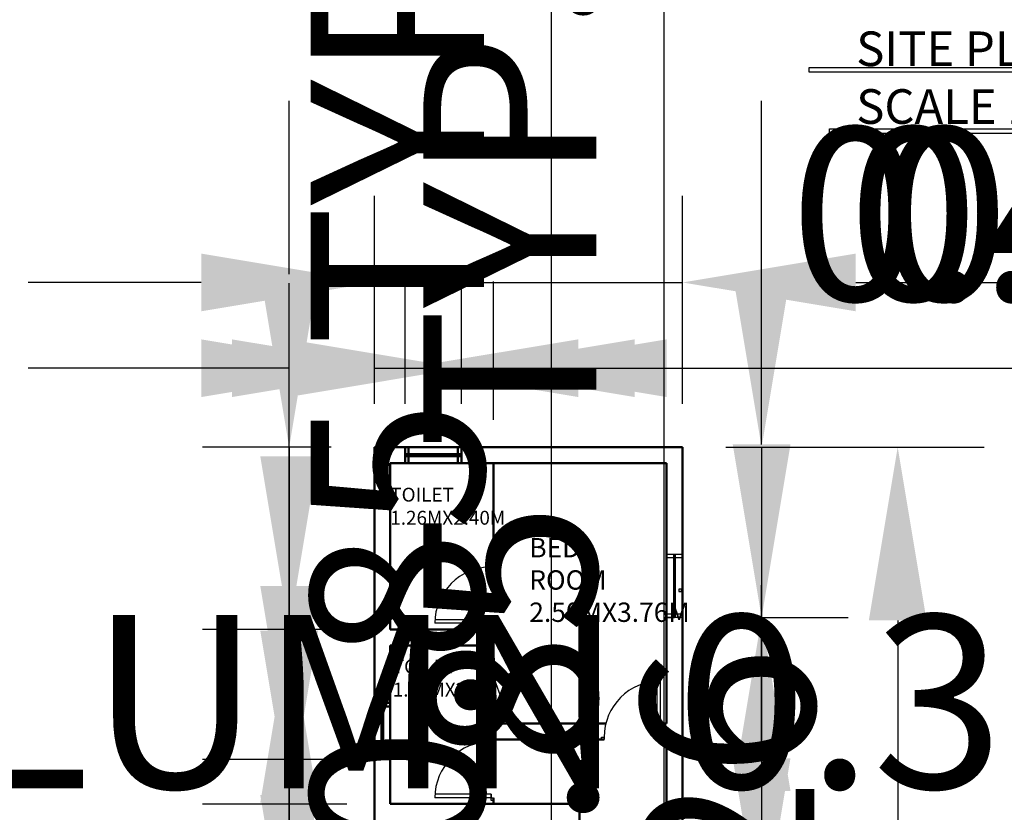
# Model space of a CAD drawing. Units: metres. Extents: x 782 to 1487, y 1262 to 7446.
# Tile 7 of 25: x 807.01 to 821.23, y 1302.06 to 1313.5. Entities that reach past the tile are written whole.
import ezdxf

# ---------------------------------------------------------------- set-up
doc = ezdxf.new("R2010")
doc.units = ezdxf.units.M
for name, color, linetype, lineweight in [('A-ANNO-DIMS', 2, 'Continuous', 18), ('A-ANNO-TEXT', 3, 'Continuous', 18), ('A-AREA-IDEN', 3, 'Continuous', 18), ('A-DOOR', 4, 'Continuous', 25), ('A-GLAZ', 4, 'Continuous', 25), ('A-WALL', 7, 'Continuous', 50), ('C-PROP', 6, 'Continuous', 25)]:
    doc.layers.add(name, color=color, linetype=linetype, lineweight=lineweight)
doc.styles.get("Standard").update_dxf_attribs({"font": 'arial.ttf'})
doc.dimstyles.new('ISO-25', dxfattribs={"dimtxt": 2.5, "dimasz": 2.5, "dimexe": 1.25, "dimexo": 0.625, "dimtad": 1, "dimtxsty": 'Standard', "dimcen": 2.5, "dimadec": 0, "dimazin": 0, "dimtfac": 1, "dimtmove": 0, "dimatfit": 3, "dimfxl": 1, "dimarcsym": 0})

# ---------------------------------------------------------------- blocks, each defined once
blk = doc.blocks.new('*D4')
at = {"layer": 'A-ANNO-DIMS', "color": 0, "lineweight": -2, "transparency": 16777216}
for p, q in [((817.205, 1307.327), (820.936, 1307.327)), ((819.686, 1304.827), (819.686, 1295.567)), ((817.205, 1293.067), (820.936, 1293.067))]:
    blk.add_line(p, q, dxfattribs=at)
at = {"layer": 'A-ANNO-DIMS', "color": 0, "transparency": 16777216}
for points in [[(819.269, 1304.827), (820.103, 1304.827), (819.686, 1307.327)], [(819.269, 1295.567), (820.103, 1295.567), (819.686, 1293.067)]]:
    blk.add_solid(points, dxfattribs=at)
at = {"layer": 'Defpoints', "color": 0, "transparency": 16777216}
for p in [(816.58, 1307.327), (816.58, 1293.067), (819.686, 1293.067)]:
    blk.add_point(p, dxfattribs=at)
at = {"layer": 'A-ANNO-DIMS', "color": 0, "transparency": 16777216, "insert": (817.558, 1300.197), "char_height": 2.5, "attachment_point": 5, "rotation": 90}
blk.add_mtext('14,26', dxfattribs=at)
blk = doc.blocks.new('*D5')
at = {"layer": 'A-ANNO-DIMS', "color": 0, "lineweight": -2, "transparency": 16777216}
for p, q in [((812.13, 1307.952), (812.13, 1310.955)), ((816.58, 1307.952), (816.58, 1310.955)), ((809.63, 1309.705), (807.13, 1309.705)), ((812.13, 1309.705), (816.58, 1309.705)), ((819.08, 1309.705), (829.443, 1309.705))]:
    blk.add_line(p, q, dxfattribs=at)
at = {"layer": 'A-ANNO-DIMS', "color": 0, "transparency": 16777216}
for points in [[(809.63, 1310.122), (809.63, 1309.289), (812.13, 1309.705)], [(819.08, 1310.122), (819.08, 1309.289), (816.58, 1309.705)]]:
    blk.add_solid(points, dxfattribs=at)
at = {"layer": 'Defpoints', "color": 0, "transparency": 16777216}
for p in [(816.58, 1309.705), (812.13, 1307.327), (816.58, 1307.327)]:
    blk.add_point(p, dxfattribs=at)
at = {"layer": 'A-ANNO-DIMS', "color": 0, "transparency": 16777216, "insert": (825.512, 1311.828), "char_height": 2.5, "attachment_point": 5}
blk.add_mtext('4,45', dxfattribs=at)
blk = doc.blocks.new('DOOR-810')
for p, q in [((0.813, 0.089), (0, 0.089)), ((0.813, 0.038), (0.813, 0.089))]:
    blk.add_line(p, q)
for points in [[(0.813, 0.851), (0.846, 0.851), (0.846, 0.89), (0.813, 0.89)], [(0.813, 0.038), (0.847, 0.038), (0.847, 0), (0.813, 0)]]:
    blk.add_lwpolyline(points, close=True)
blk.add_lwpolyline([(0.813, 0.089), (0.813, 0.038), (0, 0.038)])
blk.add_arc((0.813, 0.038), 0.813, 90, 180)
blk = doc.blocks.new('DOOR-810-C')
for p, q in [((0.801, 0.034), (0.801, 0.847)), ((0.851, 0.034), (0.801, 0.034))]:
    blk.add_line(p, q)
blk.add_lwpolyline([(0.801, 0.034), (0.851, 0.034), (0.851, 0.847)])
for points in [[(0.039, 0.034), (0.039, 0.002), (0, 0.002), (0, 0.034)], [(0.851, 0.034), (0.851, 0), (0.889, 0), (0.889, 0.034)]]:
    blk.add_lwpolyline(points, close=True)
blk.add_arc((0.851, 0.034), 0.813, 90, 180)
blk = doc.blocks.new('WIN-900-B')
for p, q in [((0, 0), (0, 0.914)), ((0, 0.914), (0.23, 0.914)), ((0.23, 0.863), (0, 0.863)), ((0.103, 0), (0.103, 0.914)), ((0.115, 0), (0.115, 0.914)), ((0.128, 0), (0.128, 0.914)), ((0.23, 0.914), (0.23, 0)), ((0.23, 0.914), (0.23, 0.863)), ((0.23, 0.051), (0, 0.051)), ((0.23, 0), (0.23, 0.051)), ((0.23, 0), (0, 0)), ((0, 0), (0.115, 0))]:
    blk.add_line(p, q)
blk.add_lwpolyline([(0.215, 0.379), (0.215, 0.412), (0.176, 0.412), (0.176, 0.379)], close=True)
blk = doc.blocks.new('*D23')
at = {"layer": 'A-ANNO-DIMS', "color": 0, "lineweight": -2, "transparency": 16777216}
for p, q in [((816.313, 1296.414), (816.313, 1315.246)), ((816.313, 1293.067), (816.313, 1293.914)), ((816.804, 1293.914), (817.563, 1293.914)), ((816.804, 1293.067), (817.563, 1293.067)), ((816.313, 1290.567), (816.313, 1288.067))]:
    blk.add_line(p, q, dxfattribs=at)
at = {"layer": 'A-ANNO-DIMS', "color": 0, "transparency": 16777216}
for points in [[(815.896, 1296.414), (816.729, 1296.414), (816.313, 1293.914)], [(815.896, 1290.567), (816.729, 1290.567), (816.313, 1293.067)]]:
    blk.add_solid(points, dxfattribs=at)
at = {"layer": 'Defpoints', "color": 0, "transparency": 16777216}
for p in [(816.179, 1293.914), (816.313, 1293.914), (816.179, 1293.067)]:
    blk.add_point(p, dxfattribs=at)
at = {"layer": 'A-ANNO-DIMS', "color": 0, "transparency": 16777216, "insert": (814.411, 1307.08), "char_height": 2.5, "attachment_point": 5, "rotation": 90}
blk.add_mtext('0.85 TYP.', dxfattribs=at)
blk = doc.blocks.new('*D24')
at = {"layer": 'A-ANNO-DIMS', "color": 0, "lineweight": -2, "transparency": 16777216}
for p, q in [((811.209, 1294.423), (808.709, 1294.423)), ((813.709, 1294.423), (814.559, 1294.423)), ((817.059, 1294.423), (852.649, 1294.423)), ((813.709, 1293.926), (813.709, 1293.173)), ((814.559, 1293.926), (814.559, 1293.173))]:
    blk.add_line(p, q, dxfattribs=at)
at = {"layer": 'A-ANNO-DIMS', "color": 0, "transparency": 16777216}
for points in [[(811.209, 1294.84), (811.209, 1294.006), (813.709, 1294.423)], [(817.059, 1294.84), (817.059, 1294.006), (814.559, 1294.423)]]:
    blk.add_solid(points, dxfattribs=at)
at = {"layer": 'Defpoints', "color": 0, "transparency": 16777216}
for p in [(813.709, 1294.551), (814.559, 1294.551), (814.559, 1294.423)]:
    blk.add_point(p, dxfattribs=at)
at = {"layer": 'A-ANNO-DIMS', "color": 0, "transparency": 16777216, "insert": (836.104, 1296.342), "char_height": 2.5, "attachment_point": 5}
blk.add_mtext('DOOR D2 0.85 TYP.', dxfattribs=at)
blk = doc.blocks.new('*D25')
at = {"layer": 'A-ANNO-DIMS', "color": 0, "lineweight": -2, "transparency": 16777216}
for p, q in [((814.687, 1297.897), (814.687, 1316.729)), ((814.687, 1294.551), (814.687, 1295.397)), ((815.184, 1295.397), (815.937, 1295.397)), ((815.184, 1294.551), (815.937, 1294.551)), ((814.687, 1292.051), (814.687, 1289.551))]:
    blk.add_line(p, q, dxfattribs=at)
at = {"layer": 'A-ANNO-DIMS', "color": 0, "transparency": 16777216}
for points in [[(814.27, 1297.897), (815.103, 1297.897), (814.687, 1295.397)], [(814.27, 1292.051), (815.103, 1292.051), (814.687, 1294.551)]]:
    blk.add_solid(points, dxfattribs=at)
at = {"layer": 'Defpoints', "color": 0, "transparency": 16777216}
for p in [(814.559, 1295.397), (814.687, 1295.397), (814.559, 1294.551)]:
    blk.add_point(p, dxfattribs=at)
at = {"layer": 'A-ANNO-DIMS', "color": 0, "transparency": 16777216, "insert": (812.785, 1308.563), "char_height": 2.5, "attachment_point": 5, "rotation": 90}
blk.add_mtext('0.85 TYP.', dxfattribs=at)
blk = doc.blocks.new('*D26')
at = {"layer": 'A-ANNO-DIMS', "color": 0, "lineweight": -2, "transparency": 16777216}
for p, q in [((828.33, 1303.223), (828.33, 1342.718)), ((828.33, 1299.809), (828.33, 1300.723)), ((828.818, 1300.723), (829.58, 1300.723)), ((828.818, 1299.809), (829.58, 1299.809)), ((828.33, 1297.309), (828.33, 1294.809))]:
    blk.add_line(p, q, dxfattribs=at)
at = {"layer": 'A-ANNO-DIMS', "color": 0, "transparency": 16777216}
for points in [[(827.913, 1303.223), (828.747, 1303.223), (828.33, 1300.723)], [(827.913, 1297.309), (828.747, 1297.309), (828.33, 1299.809)]]:
    blk.add_solid(points, dxfattribs=at)
at = {"layer": 'Defpoints', "color": 0, "transparency": 16777216}
for p in [(828.193, 1300.723), (828.33, 1300.723), (828.193, 1299.809)]:
    blk.add_point(p, dxfattribs=at)
at = {"layer": 'A-ANNO-DIMS', "color": 0, "transparency": 16777216, "insert": (826.412, 1324.22), "char_height": 2.5, "attachment_point": 5, "rotation": 90}
blk.add_mtext('WINDOW W 0.91 TYP.', dxfattribs=at)
blk = doc.blocks.new('*D30')
at = {"layer": 'A-ANNO-DIMS', "color": 0, "lineweight": -2, "transparency": 16777216}
for p, q in [((792.059, 1301.411), (789.559, 1301.411)), ((794.559, 1301.411), (794.946, 1301.411)), ((797.446, 1301.411), (832.354, 1301.411)), ((794.559, 1300.844), (794.559, 1300.161)), ((794.946, 1300.844), (794.946, 1300.161))]:
    blk.add_line(p, q, dxfattribs=at)
at = {"layer": 'A-ANNO-DIMS', "color": 0, "transparency": 16777216}
for points in [[(792.059, 1301.827), (792.059, 1300.994), (794.559, 1301.411)], [(797.446, 1301.827), (797.446, 1300.994), (794.946, 1301.411)]]:
    blk.add_solid(points, dxfattribs=at)
at = {"layer": 'Defpoints', "color": 0, "transparency": 16777216}
for p in [(794.559, 1301.469), (794.946, 1301.469), (794.946, 1301.411)]:
    blk.add_point(p, dxfattribs=at)
at = {"layer": 'A-ANNO-DIMS', "color": 0, "transparency": 16777216, "insert": (816.15, 1303.33), "char_height": 2.5, "attachment_point": 5}
blk.add_mtext('COLUMN 0.39 TYP.', dxfattribs=at)
blk = doc.blocks.new('*D43')
at = {"layer": 'A-ANNO-DIMS', "color": 0, "lineweight": -2, "transparency": 16777216}
for p, q in [((792.559, 1313.575), (792.559, 1315.72)), ((794.559, 1311.575), (794.559, 1315.72)), ((790.059, 1314.47), (787.559, 1314.47)), ((792.559, 1314.47), (794.559, 1314.47)), ((797.059, 1314.47), (807.337, 1314.47))]:
    blk.add_line(p, q, dxfattribs=at)
at = {"layer": 'A-ANNO-DIMS', "color": 0, "transparency": 16777216}
for points in [[(790.059, 1314.887), (790.059, 1314.054), (792.559, 1314.47)], [(797.059, 1314.887), (797.059, 1314.054), (794.559, 1314.47)]]:
    blk.add_solid(points, dxfattribs=at)
at = {"layer": 'Defpoints', "color": 0, "transparency": 16777216}
for p in [(794.559, 1314.47), (792.559, 1312.95), (794.559, 1310.95)]:
    blk.add_point(p, dxfattribs=at)
at = {"layer": 'A-ANNO-DIMS', "color": 0, "transparency": 16777216, "insert": (803.448, 1316.372), "char_height": 2.5, "attachment_point": 5}
blk.add_mtext('2.00', dxfattribs=at)
blk = doc.blocks.new('*D44')
at = {"layer": 'A-ANNO-DIMS', "color": 0, "lineweight": -2, "transparency": 16777216}
for p, q in [((800.039, 1311.575), (800.039, 1315.72)), ((801.429, 1313.575), (801.429, 1315.72)), ((797.539, 1314.47), (795.039, 1314.47)), ((800.039, 1314.47), (801.429, 1314.47)), ((803.929, 1314.47), (813.943, 1314.47))]:
    blk.add_line(p, q, dxfattribs=at)
at = {"layer": 'A-ANNO-DIMS', "color": 0, "transparency": 16777216}
for points in [[(797.539, 1314.887), (797.539, 1314.054), (800.039, 1314.47)], [(803.929, 1314.887), (803.929, 1314.054), (801.429, 1314.47)]]:
    blk.add_solid(points, dxfattribs=at)
at = {"layer": 'Defpoints', "color": 0, "transparency": 16777216}
for p in [(801.429, 1314.47), (801.429, 1312.95), (800.039, 1310.95)]:
    blk.add_point(p, dxfattribs=at)
at = {"layer": 'A-ANNO-DIMS', "color": 0, "transparency": 16777216, "insert": (810.186, 1316.373), "char_height": 2.5, "attachment_point": 5}
blk.add_mtext('1.39', dxfattribs=at)
blk = doc.blocks.new('*D53')
at = {"layer": 'A-ANNO-DIMS', "color": 0, "lineweight": -2, "transparency": 16777216}
for p, q in [((810.9, 1309.827), (810.9, 1312.327)), ((811.505, 1307.327), (809.65, 1307.327)), ((810.9, 1307.327), (810.9, 1304.697)), ((811.735, 1304.697), (809.65, 1304.697)), ((810.9, 1302.197), (810.9, 1291.911))]:
    blk.add_line(p, q, dxfattribs=at)
at = {"layer": 'A-ANNO-DIMS', "color": 0, "transparency": 16777216}
for points in [[(810.483, 1309.827), (811.317, 1309.827), (810.9, 1307.327)], [(810.483, 1302.197), (811.317, 1302.197), (810.9, 1304.697)]]:
    blk.add_solid(points, dxfattribs=at)
at = {"layer": 'Defpoints', "color": 0, "transparency": 16777216}
for p in [(812.13, 1307.327), (810.9, 1304.697), (812.36, 1304.697)]:
    blk.add_point(p, dxfattribs=at)
at = {"layer": 'A-ANNO-DIMS', "color": 0, "transparency": 16777216, "insert": (808.998, 1295.804), "char_height": 2.5, "attachment_point": 5, "rotation": 90}
blk.add_mtext('2.63', dxfattribs=at)
blk = doc.blocks.new('*D54')
at = {"layer": 'A-ANNO-DIMS', "color": 0, "lineweight": -2, "transparency": 16777216}
for p, q in [((810.9, 1307.197), (810.9, 1309.697)), ((811.735, 1304.697), (809.65, 1304.697)), ((810.9, 1304.697), (810.9, 1302.822)), ((811.503, 1302.822), (809.65, 1302.822)), ((810.9, 1300.322), (810.9, 1290.308))]:
    blk.add_line(p, q, dxfattribs=at)
at = {"layer": 'A-ANNO-DIMS', "color": 0, "transparency": 16777216}
for points in [[(810.483, 1307.197), (811.317, 1307.197), (810.9, 1304.697)], [(810.483, 1300.322), (811.317, 1300.322), (810.9, 1302.822)]]:
    blk.add_solid(points, dxfattribs=at)
at = {"layer": 'Defpoints', "color": 0, "transparency": 16777216}
for p in [(812.36, 1304.697), (810.9, 1302.822), (812.128, 1302.822)]:
    blk.add_point(p, dxfattribs=at)
at = {"layer": 'A-ANNO-DIMS', "color": 0, "transparency": 16777216, "insert": (808.999, 1294.065), "char_height": 2.5, "attachment_point": 5, "rotation": 90}
blk.add_mtext('1.88', dxfattribs=at)
blk = doc.blocks.new('*D55')
at = {"layer": 'A-ANNO-DIMS', "color": 0, "lineweight": -2, "transparency": 16777216}
for p, q in [((810.9, 1305.322), (810.9, 1307.822)), ((811.503, 1302.822), (809.65, 1302.822)), ((810.9, 1302.822), (810.9, 1302.177)), ((811.735, 1302.177), (809.65, 1302.177)), ((810.9, 1299.677), (810.9, 1289.444))]:
    blk.add_line(p, q, dxfattribs=at)
at = {"layer": 'A-ANNO-DIMS', "color": 0, "transparency": 16777216}
for points in [[(810.483, 1305.322), (811.317, 1305.322), (810.9, 1302.822)], [(810.483, 1299.677), (811.317, 1299.677), (810.9, 1302.177)]]:
    blk.add_solid(points, dxfattribs=at)
at = {"layer": 'Defpoints', "color": 0, "transparency": 16777216}
for p in [(812.128, 1302.822), (810.9, 1302.177), (812.36, 1302.177)]:
    blk.add_point(p, dxfattribs=at)
at = {"layer": 'A-ANNO-DIMS', "color": 0, "transparency": 16777216, "insert": (808.999, 1293.311), "char_height": 2.5, "attachment_point": 5, "rotation": 90}
blk.add_mtext('0.64', dxfattribs=at)
blk = doc.blocks.new('*D56')
at = {"layer": 'A-ANNO-DIMS', "color": 0, "lineweight": -2, "transparency": 16777216}
for p, q in [((810.9, 1304.677), (810.9, 1307.177)), ((811.735, 1302.177), (809.65, 1302.177)), ((810.9, 1302.177), (810.9, 1299.809)), ((811.505, 1299.809), (809.65, 1299.809)), ((810.9, 1297.309), (810.9, 1287.022))]:
    blk.add_line(p, q, dxfattribs=at)
at = {"layer": 'A-ANNO-DIMS', "color": 0, "transparency": 16777216}
for points in [[(810.483, 1304.677), (811.317, 1304.677), (810.9, 1302.177)], [(810.483, 1297.309), (811.317, 1297.309), (810.9, 1299.809)]]:
    blk.add_solid(points, dxfattribs=at)
at = {"layer": 'Defpoints', "color": 0, "transparency": 16777216}
for p in [(812.36, 1302.177), (810.9, 1299.809), (812.13, 1299.809)]:
    blk.add_point(p, dxfattribs=at)
at = {"layer": 'A-ANNO-DIMS', "color": 0, "transparency": 16777216, "insert": (808.998, 1290.916), "char_height": 2.5, "attachment_point": 5, "rotation": 90}
blk.add_mtext('2.37', dxfattribs=at)
blk = doc.blocks.new('*D57')
at = {"layer": 'A-ANNO-DIMS', "color": 0, "lineweight": -2, "transparency": 16777216}
for p, q in [((810.9, 1302.309), (810.9, 1304.809)), ((811.505, 1299.809), (809.65, 1299.809)), ((810.9, 1299.809), (810.9, 1298.647)), ((811.735, 1298.647), (809.65, 1298.647)), ((810.9, 1296.147), (810.9, 1286.141))]:
    blk.add_line(p, q, dxfattribs=at)
at = {"layer": 'A-ANNO-DIMS', "color": 0, "transparency": 16777216}
for points in [[(810.483, 1302.309), (811.317, 1302.309), (810.9, 1299.809)], [(810.483, 1296.147), (811.317, 1296.147), (810.9, 1298.647)]]:
    blk.add_solid(points, dxfattribs=at)
at = {"layer": 'Defpoints', "color": 0, "transparency": 16777216}
for p in [(812.13, 1299.809), (810.9, 1298.647), (812.36, 1298.647)]:
    blk.add_point(p, dxfattribs=at)
at = {"layer": 'A-ANNO-DIMS', "color": 0, "transparency": 16777216, "insert": (808.999, 1289.894), "char_height": 2.5, "attachment_point": 5, "rotation": 90}
blk.add_mtext('1.16', dxfattribs=at)
blk = doc.blocks.new('*D58')
at = {"layer": 'A-ANNO-DIMS', "color": 0, "lineweight": -2, "transparency": 16777216}
for p, q in [((810.9, 1301.147), (810.9, 1303.647)), ((811.735, 1298.647), (809.65, 1298.647)), ((810.9, 1298.647), (810.9, 1296.5)), ((811.507, 1296.5), (809.65, 1296.5)), ((810.9, 1294), (810.9, 1281.772))]:
    blk.add_line(p, q, dxfattribs=at)
at = {"layer": 'A-ANNO-DIMS', "color": 0, "transparency": 16777216}
for points in [[(810.483, 1301.147), (811.317, 1301.147), (810.9, 1298.647)], [(810.483, 1294), (811.317, 1294), (810.9, 1296.5)]]:
    blk.add_solid(points, dxfattribs=at)
at = {"layer": 'Defpoints', "color": 0, "transparency": 16777216}
for p in [(812.36, 1298.647), (810.9, 1296.5), (812.132, 1296.5)]:
    blk.add_point(p, dxfattribs=at)
at = {"layer": 'A-ANNO-DIMS', "color": 0, "transparency": 16777216, "insert": (809.02, 1286.636), "char_height": 2.5, "attachment_point": 5, "rotation": 90}
blk.add_mtext('2.147', dxfattribs=at)
blk = doc.blocks.new('*D63')
at = {"layer": 'A-ANNO-DIMS', "color": 0, "lineweight": -2, "transparency": 16777216}
for p, q in [((817.721, 1309.827), (817.721, 1312.327)), ((817.205, 1307.327), (818.971, 1307.327)), ((817.721, 1307.327), (817.721, 1304.867)), ((817.205, 1304.867), (818.971, 1304.867)), ((817.721, 1302.367), (817.721, 1292.082))]:
    blk.add_line(p, q, dxfattribs=at)
at = {"layer": 'A-ANNO-DIMS', "color": 0, "transparency": 16777216}
for points in [[(817.304, 1309.827), (818.138, 1309.827), (817.721, 1307.327)], [(817.304, 1302.367), (818.138, 1302.367), (817.721, 1304.867)]]:
    blk.add_solid(points, dxfattribs=at)
at = {"layer": 'Defpoints', "color": 0, "transparency": 16777216}
for p in [(816.58, 1307.327), (816.58, 1304.867), (817.721, 1304.867)]:
    blk.add_point(p, dxfattribs=at)
at = {"layer": 'A-ANNO-DIMS', "color": 0, "transparency": 16777216, "insert": (815.82, 1295.974), "char_height": 2.5, "attachment_point": 5, "rotation": 90}
blk.add_mtext('2.46', dxfattribs=at)
blk = doc.blocks.new('*D64')
at = {"layer": 'A-ANNO-DIMS', "color": 0, "lineweight": -2, "transparency": 16777216}
for p, q in [((817.721, 1307.367), (817.721, 1309.867)), ((817.205, 1304.867), (818.971, 1304.867)), ((817.721, 1304.867), (817.721, 1300.338)), ((817.206, 1300.338), (818.971, 1300.338)), ((817.721, 1297.838), (817.721, 1285.546))]:
    blk.add_line(p, q, dxfattribs=at)
at = {"layer": 'A-ANNO-DIMS', "color": 0, "transparency": 16777216}
for points in [[(817.304, 1307.367), (818.138, 1307.367), (817.721, 1304.867)], [(817.304, 1297.838), (818.138, 1297.838), (817.721, 1300.338)]]:
    blk.add_solid(points, dxfattribs=at)
at = {"layer": 'Defpoints', "color": 0, "transparency": 16777216}
for p in [(816.58, 1304.867), (816.581, 1300.338), (817.721, 1300.338)]:
    blk.add_point(p, dxfattribs=at)
at = {"layer": 'A-ANNO-DIMS', "color": 0, "transparency": 16777216, "insert": (815.82, 1290.442), "char_height": 2.5, "attachment_point": 5, "rotation": 90}
blk.add_mtext('4.529', dxfattribs=at)
blk = doc.blocks.new('*D65')
at = {"layer": 'A-ANNO-DIMS', "color": 0, "lineweight": -2, "transparency": 16777216}
for p, q in [((817.721, 1302.838), (817.721, 1305.338)), ((817.206, 1300.338), (818.971, 1300.338)), ((817.721, 1300.338), (817.721, 1296.196)), ((817.205, 1296.196), (818.971, 1296.196)), ((817.721, 1293.696), (817.721, 1281.435))]:
    blk.add_line(p, q, dxfattribs=at)
at = {"layer": 'A-ANNO-DIMS', "color": 0, "transparency": 16777216}
for points in [[(817.304, 1302.838), (818.138, 1302.838), (817.721, 1300.338)], [(817.304, 1293.696), (818.138, 1293.696), (817.721, 1296.196)]]:
    blk.add_solid(points, dxfattribs=at)
at = {"layer": 'Defpoints', "color": 0, "transparency": 16777216}
for p in [(816.581, 1300.338), (816.58, 1296.196), (817.721, 1296.196)]:
    blk.add_point(p, dxfattribs=at)
at = {"layer": 'A-ANNO-DIMS', "color": 0, "transparency": 16777216, "insert": (815.841, 1286.315), "char_height": 2.5, "attachment_point": 5, "rotation": 90}
blk.add_mtext('4.142', dxfattribs=at)
blk = doc.blocks.new('*D70')
at = {"layer": 'A-ANNO-DIMS', "color": 0, "lineweight": -2, "transparency": 16777216}
for p, q in [((812.13, 1307.952), (812.13, 1309.718)), ((812.573, 1307.953), (812.573, 1309.718)), ((809.63, 1308.468), (807.13, 1308.468)), ((812.13, 1308.468), (812.573, 1308.468)), ((815.073, 1308.468), (825.307, 1308.468))]:
    blk.add_line(p, q, dxfattribs=at)
at = {"layer": 'A-ANNO-DIMS', "color": 0, "transparency": 16777216}
for points in [[(809.63, 1308.884), (809.63, 1308.051), (812.13, 1308.468)], [(815.073, 1308.884), (815.073, 1308.051), (812.573, 1308.468)]]:
    blk.add_solid(points, dxfattribs=at)
at = {"layer": 'Defpoints', "color": 0, "transparency": 16777216}
for p in [(812.573, 1308.468), (812.13, 1307.327), (812.573, 1307.328)]:
    blk.add_point(p, dxfattribs=at)
at = {"layer": 'A-ANNO-DIMS', "color": 0, "transparency": 16777216, "insert": (821.44, 1310.369), "char_height": 2.5, "attachment_point": 5}
blk.add_mtext('0.44', dxfattribs=at)
blk = doc.blocks.new('*D71')
at = {"layer": 'A-ANNO-DIMS', "color": 0, "lineweight": -2, "transparency": 16777216}
for p, q in [((812.573, 1307.953), (812.573, 1309.718)), ((813.387, 1307.953), (813.387, 1309.718)), ((810.073, 1308.468), (807.573, 1308.468)), ((812.573, 1308.468), (813.387, 1308.468)), ((815.887, 1308.468), (828.063, 1308.468))]:
    blk.add_line(p, q, dxfattribs=at)
at = {"layer": 'A-ANNO-DIMS', "color": 0, "transparency": 16777216}
for points in [[(810.073, 1308.884), (810.073, 1308.051), (812.573, 1308.468)], [(815.887, 1308.884), (815.887, 1308.051), (813.387, 1308.468)]]:
    blk.add_solid(points, dxfattribs=at)
at = {"layer": 'Defpoints', "color": 0, "transparency": 16777216}
for p in [(813.387, 1308.468), (812.573, 1307.328), (813.387, 1307.328)]:
    blk.add_point(p, dxfattribs=at)
at = {"layer": 'A-ANNO-DIMS', "color": 0, "transparency": 16777216, "insert": (823.225, 1310.369), "char_height": 2.5, "attachment_point": 5}
blk.add_mtext('0.814', dxfattribs=at)
blk = doc.blocks.new('*D72')
at = {"layer": 'A-ANNO-DIMS', "color": 0, "lineweight": -2, "transparency": 16777216}
for p, q in [((813.387, 1307.953), (813.387, 1309.718)), ((813.85, 1307.722), (813.85, 1309.718)), ((810.887, 1308.468), (808.387, 1308.468)), ((813.387, 1308.468), (813.85, 1308.468)), ((816.35, 1308.468), (826.592, 1308.468))]:
    blk.add_line(p, q, dxfattribs=at)
at = {"layer": 'A-ANNO-DIMS', "color": 0, "transparency": 16777216}
for points in [[(810.887, 1308.884), (810.887, 1308.051), (813.387, 1308.468)], [(816.35, 1308.884), (816.35, 1308.051), (813.85, 1308.468)]]:
    blk.add_solid(points, dxfattribs=at)
at = {"layer": 'Defpoints', "color": 0, "transparency": 16777216}
for p in [(813.85, 1308.468), (813.387, 1307.328), (813.85, 1307.097)]:
    blk.add_point(p, dxfattribs=at)
at = {"layer": 'A-ANNO-DIMS', "color": 0, "transparency": 16777216, "insert": (822.721, 1310.369), "char_height": 2.5, "attachment_point": 5}
blk.add_mtext('0.46', dxfattribs=at)

msp = doc.modelspace()

# ---------------------------------------------------------------- linework, layer by layer
at = {"layer": 'A-WALL'}
for p, q in [((812.13, 1304.6974), (812.13, 1307.3274)), ((812.13, 1307.3274), (813.62, 1307.3274)), ((812.5733, 1307.3276), (813.3873, 1307.3276)), ((812.5733, 1307.0976), (812.5733, 1307.3276)), ((812.5733, 1307.3276), (812.5733, 1307.2126)), ((812.6241, 1307.0976), (812.6241, 1307.3276)), ((813.3365, 1307.0976), (813.3365, 1307.3276)), ((813.3873, 1307.3276), (813.3873, 1307.0976)), ((813.62, 1307.3274), (816.58, 1307.3274)), ((816.58, 1307.3274), (816.58, 1303.3374)), ((812.5733, 1307.2253), (813.3873, 1307.2253)), ((812.5733, 1307.2126), (813.3873, 1307.2126)), ((812.5733, 1307.1999), (813.3873, 1307.1999)), ((812.36, 1304.6974), (812.36, 1307.0974)), ((812.36, 1307.0974), (816.35, 1307.0974)), ((813.3873, 1307.0976), (812.5733, 1307.0976)), ((812.5733, 1307.0976), (812.6241, 1307.0976)), ((813.3873, 1307.0976), (813.3365, 1307.0976)), ((813.85, 1307.0974), (813.85, 1305.5981)), ((813.85, 1307.0974), (816.35, 1307.0974)), ((813.85, 1305.5981), (813.85, 1307.0974)), ((816.35, 1307.0974), (816.35, 1303.3374)), ((813.85, 1303.3374), (813.85, 1304.786)), ((813.85, 1304.786), (813.85, 1304.6974)), ((813.85, 1304.6974), (813.85, 1304.7482)), ((812.13, 1302.1774), (812.13, 1304.6974)), ((812.36, 1304.6974), (813.62, 1304.6974)), ((813.62, 1304.6974), (813.85, 1304.6974)), ((812.36, 1302.1774), (812.36, 1304.4674)), ((812.36, 1304.4674), (813.62, 1304.4674)), ((812.36, 1304.4674), (813.62, 1304.4674)), ((813.62, 1304.4674), (813.62, 1303.0548)), ((813.62, 1303.3374), (813.62, 1304.4674)), ((813.62, 1304.4674), (813.85, 1304.4674)), ((813.85, 1304.4674), (813.85, 1304.4166)), ((812.1285, 1302.8221), (812.1285, 1303.6361)), ((812.1285, 1303.6361), (812.3585, 1303.6361)), ((812.1285, 1303.6361), (812.1285, 1303.5853)), ((812.1285, 1303.5853), (812.3585, 1303.5853)), ((812.2308, 1303.6361), (812.2308, 1302.8221)), ((812.3585, 1303.6361), (812.2435, 1303.6361)), ((812.2435, 1303.6361), (812.2435, 1302.8221)), ((812.2562, 1303.6361), (812.2562, 1302.8221)), ((812.3585, 1303.6361), (812.3585, 1302.8221)), ((815.4726, 1303.3374), (813.85, 1303.3374)), ((816.35, 1303.3374), (816.2614, 1303.3374)), ((816.58, 1303.3374), (816.58, 1293.0674)), ((815.4493, 1303.1074), (813.85, 1303.1074)), ((816.35, 1303.1074), (816.2614, 1303.1074)), ((816.35, 1303.1074), (816.2992, 1303.1074)), ((816.35, 1303.1074), (816.35, 1298.6474)), ((812.1285, 1302.8221), (812.1285, 1302.8729)), ((812.1285, 1302.8729), (812.3585, 1302.8729)), ((812.3585, 1302.8221), (812.1285, 1302.8221)), ((812.13, 1298.6474), (812.13, 1302.1774)), ((812.36, 1302.1774), (815.09, 1302.1774)), ((813.85, 1302.266), (813.85, 1302.1774)), ((813.85, 1302.1774), (813.85, 1302.2282)), ((815.09, 1302.1774), (815.09, 1299.5481))]:
    msp.add_line(p, q, dxfattribs=at)
at = {"layer": 'C-PROP'}
for p, q in [((818.4097, 1312.8097), (823.558, 1312.8097)), ((818.4097, 1312.7398), (818.4097, 1312.8097)), ((823.558, 1312.7398), (818.4097, 1312.7398)), ((818.7034, 1311.923), (823.8517, 1311.923)), ((818.7034, 1311.8532), (818.7034, 1311.923)), ((823.8517, 1311.8532), (818.7034, 1311.8532))]:
    msp.add_line(p, q, dxfattribs=at)

# ---------------------------------------------------------------- block references
at = {"layer": 'A-DOOR'}
for name, p in [('DOOR-810', (813.003, 1304.748)), ('DOOR-810-C', (815.41, 1303.107)), ('DOOR-810', (813.003, 1302.228))]:
    msp.add_blockref(name, p, dxfattribs=at)
at = {"layer": 'A-GLAZ'}
msp.add_blockref('WIN-900-B', (816.35, 1304.867), dxfattribs=at)

# ---------------------------------------------------------------- texts
at = {"layer": 'A-ANNO-TEXT', "insert": (819.087, 1314.1616), "char_height": 0.5, "attachment_point": 1}
msp.add_mtext_dynamic_manual_height_columns('\\PSITE PLAN\\PSCALE 1:200', width=6.191207, gutter_width=12.5, heights=[0], dxfattribs=at)
at = {"layer": 'A-AREA-IDEN', "attachment_point": 1}
for s, width, gutter_width, insert, char_height in [('\\P{\\H0.4x;TOILET\\P1.26MX2.40M}', 1.153085, 12.5, (812.36, 1307.5758), 0.5), ('BED ROOM\\P2.50MX3.76M', 0.64421, 6.9836, (814.3665, 1306.0163), 0.279342), ('\\P{\\H0.4x;TOILET\\P1.26MX2.40M}', 1.153085, 12.5, (812.3959, 1305.0951), 0.5)]:
    msp.add_mtext_dynamic_manual_height_columns(s, width=width, gutter_width=gutter_width, heights=[0], dxfattribs=dict(at, insert=insert, char_height=char_height))

# ---------------------------------------------------------------- dimensions: what is measured, and where the dimension line sits
at = {"layer": 'A-ANNO-DIMS'}
for base, p1, p2, text, picture, middle in [((828.3302, 1300.7228), (828.1931, 1299.8088), (828.1931, 1300.7228), 'WINDOW W <> TYP.', '*D26', (826.4117, 1324.2204)), ((814.6868, 1295.3974), (814.5592, 1294.5507), (814.5592, 1295.3974), '<> TYP.', '*D25', (812.7854, 1308.5633)), ((816.3126, 1293.9141), (816.1792, 1293.0674), (816.1792, 1293.9141), '<> TYP.', '*D23', (814.4112, 1307.08))]:
    dim = msp.add_linear_dim(base=base, p1=p1, p2=p2, angle=90, text=text, dimstyle='ISO-25', override={"dimdec": 2, "dimlfac": 1, "dimrnd": 0, "dimzin": 0, "dimdsep": 46, "dimlunit": 2}, dxfattribs=at)
    dim.commit()
    dim.dimension.update_dxf_attribs({"geometry": picture, "text_midpoint": middle})
for base, p1, p2, override, picture, middle in [((794.559, 1314.4703), (792.559, 1312.9503), (794.559, 1310.9503), {"dimdec": 2, "dimlfac": 1, "dimrnd": 0, "dimzin": 0, "dimdsep": 46, "dimlunit": 2}, '*D43', (803.448, 1316.3718)), ((801.429, 1314.4703), (800.039, 1310.9503), (801.429, 1312.9503), {"dimdec": 2, "dimlfac": 1, "dimrnd": 0, "dimzin": 0, "dimdsep": 46, "dimlunit": 2}, '*D44', (810.1859, 1316.3726)), ((816.58, 1309.7054), (812.13, 1307.3274), (816.58, 1307.3274), {"dimclrd": 0, "dimclre": 0, "dimclrt": 0}, '*D5', (825.5116, 1311.8277)), ((812.5733, 1308.4676), (812.13, 1307.3274), (812.5733, 1307.3276), {"dimdec": 2, "dimlfac": 1, "dimrnd": 0, "dimzin": 0, "dimdsep": 46, "dimlunit": 2}, '*D70', (821.4401, 1310.369)), ((813.3873, 1308.4676), (812.5733, 1307.3276), (813.3873, 1307.3276), {"dimdec": 3, "dimlfac": 1, "dimrnd": 0, "dimzin": 0, "dimdsep": 46, "dimlunit": 2}, '*D71', (823.2253, 1310.369)), ((813.85, 1308.4676), (813.3873, 1307.3276), (813.85, 1307.0974), {"dimdec": 2, "dimlfac": 1, "dimrnd": 0, "dimzin": 0, "dimdsep": 46, "dimlunit": 2}, '*D72', (822.7211, 1310.369))]:
    dim = msp.add_linear_dim(base=base, p1=p1, p2=p2, dimstyle='ISO-25', override=override, dxfattribs=at)
    dim.commit()
    dim.dimension.update_dxf_attribs({"geometry": picture, "text_midpoint": middle})
for base, p1, p2, override, picture, middle in [((810.9, 1304.6974), (812.13, 1307.3274), (812.36, 1304.6974), {"dimdec": 2, "dimlfac": 1, "dimrnd": 0, "dimzin": 0, "dimdsep": 46, "dimlunit": 2}, '*D53', (808.9978, 1295.8042)), ((817.7211, 1304.8669), (816.58, 1307.3274), (816.5802, 1304.8669), {"dimdec": 2, "dimlfac": 1, "dimrnd": 0, "dimzin": 0, "dimdsep": 46, "dimlunit": 2}, '*D63', (815.8196, 1295.9745)), ((817.7211, 1300.3378), (816.5802, 1304.8669), (816.5811, 1300.3378), {"dimdec": 3, "dimlfac": 1, "dimrnd": 0, "dimzin": 0, "dimdsep": 46, "dimlunit": 2}, '*D64', (815.8196, 1290.4419)), ((810.9, 1302.8221), (812.36, 1304.6974), (812.1285, 1302.8221), {"dimdec": 2, "dimlfac": 1, "dimrnd": 0, "dimzin": 0, "dimdsep": 46, "dimlunit": 2}, '*D54', (808.9986, 1294.0652)), ((810.9, 1302.1774), (812.1285, 1302.8221), (812.36, 1302.1774), {"dimdec": 2, "dimlfac": 1, "dimrnd": 0, "dimzin": 0, "dimdsep": 46, "dimlunit": 2}, '*D55', (808.9986, 1293.3106)), ((819.6859, 1293.0674), (816.58, 1307.3274), (816.58, 1293.0674), {"dimclrd": 0, "dimclre": 0, "dimclrt": 0}, '*D4', (817.5585, 1300.1974)), ((810.9, 1299.8088), (812.36, 1302.1774), (812.1301, 1299.8088), {"dimdec": 2, "dimlfac": 1, "dimrnd": 0, "dimzin": 0, "dimdsep": 46, "dimlunit": 2}, '*D56', (808.9978, 1290.9156)), ((817.7211, 1296.196), (816.5811, 1300.3378), (816.58, 1296.196), {"dimdec": 3, "dimlfac": 1, "dimrnd": 0, "dimzin": 0, "dimdsep": 46, "dimlunit": 2}, '*D65', (815.8409, 1286.3153)), ((810.9, 1298.6474), (812.1301, 1299.8088), (812.36, 1298.6474), {"dimdec": 2, "dimlfac": 1, "dimrnd": 0, "dimzin": 0, "dimdsep": 46, "dimlunit": 2}, '*D57', (808.9986, 1289.894)), ((810.9, 1296.5004), (812.36, 1298.6474), (812.1317, 1296.5004), {"dimdec": 3, "dimlfac": 1, "dimrnd": 0, "dimzin": 0, "dimdsep": 46, "dimlunit": 2}, '*D58', (809.0199, 1286.636))]:
    dim = msp.add_linear_dim(base=base, p1=p1, p2=p2, angle=90, dimstyle='ISO-25', override=override, dxfattribs=at)
    dim.commit()
    dim.dimension.update_dxf_attribs({"geometry": picture, "text_midpoint": middle})
for base, p1, p2, text, picture, middle in [((794.9459, 1301.4107), (794.559, 1301.4687), (794.9459, 1301.4687), 'COLUMN <> TYP.', '*D30', (816.1499, 1303.33)), ((814.5592, 1294.4231), (813.7086, 1294.5507), (814.5592, 1294.5507), 'DOOR D2 <> TYP.', '*D24', (836.1042, 1296.3416))]:
    dim = msp.add_linear_dim(base=base, p1=p1, p2=p2, text=text, dimstyle='ISO-25', override={"dimdec": 2, "dimlfac": 1, "dimrnd": 0, "dimzin": 0, "dimdsep": 46, "dimlunit": 2}, dxfattribs=at)
    dim.commit()
    dim.dimension.update_dxf_attribs({"geometry": picture, "text_midpoint": middle})

doc.saveas('drawing.dxf')
